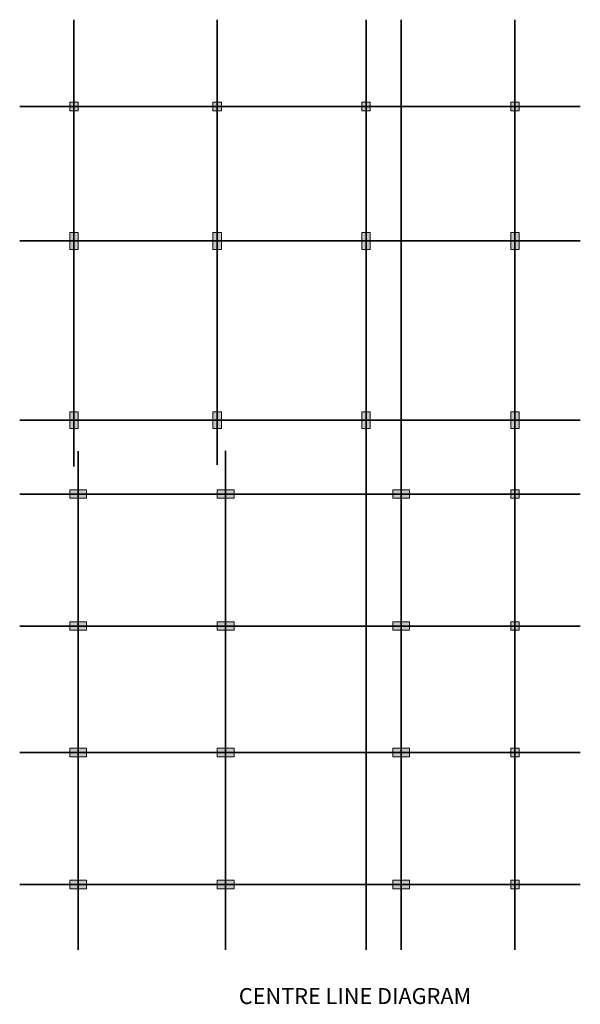
# Model space of a CAD drawing. Units: inches. Extents: x 9239 to 26065, y 6728 to 14611.
# Tile 6 of 12: x 12020 to 12619, y 6917 to 7969. Entities that reach past the tile are written whole.
import ezdxf

# ---------------------------------------------------------------- set-up
doc = ezdxf.new("R2010")
doc.units = ezdxf.units.IN
doc.header["$MEASUREMENT"] = 0
doc.linetypes.add('CENTER', pattern=[50.8, 31.75, -6.35, 6.35, -6.35])
for name, color, linetype, lineweight in [('A-ANNO-TEXT', 7, 'Continuous', 18), ('A-GRID', 3, 'CENTER', 18), ('S-COLS', 1, 'Continuous', 35), ('S-PATT', 252, 'Continuous', 13)]:
    doc.layers.add(name, color=color, linetype=linetype, lineweight=lineweight)
doc.styles.get("Standard").update_dxf_attribs({"font": 'arial.ttf'})

msp = doc.modelspace()

# ---------------------------------------------------------------- hatches: boundary and pattern name
at = {"layer": 'S-PATT'}
h = msp.add_hatch(color=256, dxfattribs=at)
h.dxf.hatch_style = 1
h.paths.add_polyline_path([(12082.24, 7880.66), (12077.74, 7880.66), (12077.74, 7876.16), (12082.24, 7876.16)])
h.paths.add_polyline_path([(12077.74, 7880.66), (12073.24, 7880.66), (12073.24, 7876.16), (12077.74, 7876.16)])
h.paths.add_polyline_path([(12077.74, 7876.16), (12073.24, 7876.16), (12073.24, 7871.66), (12077.74, 7871.66)])
h.paths.add_polyline_path([(12082.24, 7876.16), (12077.74, 7876.16), (12077.74, 7871.66), (12082.24, 7871.66)])
h.paths.add_polyline_path([(12235.24, 7880.66), (12230.74, 7880.66), (12230.74, 7876.16), (12235.24, 7876.16)])
h.paths.add_polyline_path([(12235.24, 7876.16), (12230.74, 7876.16), (12230.74, 7871.66), (12235.24, 7871.66)])
h.paths.add_polyline_path([(12230.74, 7876.16), (12226.24, 7876.16), (12226.24, 7871.66), (12230.74, 7871.66)])
h.paths.add_polyline_path([(12230.74, 7880.66), (12226.24, 7880.66), (12226.24, 7876.16), (12230.74, 7876.16)])
h.paths.add_polyline_path([(12394.24, 7876.16), (12389.74, 7876.16), (12389.74, 7871.66), (12394.24, 7871.66)])
h.paths.add_polyline_path([(12394.24, 7880.66), (12389.74, 7880.66), (12389.74, 7876.16), (12394.24, 7876.16)])
h.paths.add_polyline_path([(12389.74, 7880.66), (12385.24, 7880.66), (12385.24, 7876.16), (12389.74, 7876.16)])
h.paths.add_polyline_path([(12389.74, 7876.16), (12385.24, 7876.16), (12385.24, 7871.66), (12389.74, 7871.66)])
h.paths.add_polyline_path([(12553.24, 7880.66), (12548.74, 7880.66), (12548.74, 7876.16), (12553.24, 7876.16)])
h.paths.add_polyline_path([(12548.74, 7880.66), (12544.24, 7880.66), (12544.24, 7876.16), (12548.74, 7876.16)])
h.paths.add_polyline_path([(12548.74, 7876.16), (12544.24, 7876.16), (12544.24, 7871.66), (12548.74, 7871.66)])
h.paths.add_polyline_path([(12553.24, 7876.16), (12548.74, 7876.16), (12548.74, 7871.66), (12553.24, 7871.66)])
h.paths.add_polyline_path([(12553.24, 7732.59), (12548.74, 7732.59), (12548.74, 7723.59), (12553.24, 7723.59)])
h.paths.add_polyline_path([(12553.24, 7741.59), (12548.74, 7741.59), (12548.74, 7732.59), (12553.24, 7732.59)])
h.paths.add_polyline_path([(12548.74, 7741.59), (12544.24, 7741.59), (12544.24, 7732.59), (12548.74, 7732.59)])
h.paths.add_polyline_path([(12548.74, 7732.59), (12544.24, 7732.59), (12544.24, 7723.59), (12548.74, 7723.59)])
h.paths.add_polyline_path([(12394.24, 7741.59), (12389.74, 7741.59), (12389.74, 7732.59), (12394.24, 7732.59)])
h.paths.add_polyline_path([(12389.74, 7741.59), (12385.24, 7741.59), (12385.24, 7732.59), (12389.74, 7732.59)])
h.paths.add_polyline_path([(12389.74, 7732.59), (12385.24, 7732.59), (12385.24, 7723.59), (12389.74, 7723.59)])
h.paths.add_polyline_path([(12394.24, 7732.59), (12389.74, 7732.59), (12389.74, 7723.59), (12394.24, 7723.59)])
h.paths.add_polyline_path([(12230.74, 7741.59), (12226.24, 7741.59), (12226.24, 7732.59), (12230.74, 7732.59)])
h.paths.add_polyline_path([(12235.24, 7741.59), (12230.74, 7741.59), (12230.74, 7732.59), (12235.24, 7732.59)])
h.paths.add_polyline_path([(12235.24, 7732.59), (12230.74, 7732.59), (12230.74, 7723.59), (12235.24, 7723.59)])
h.paths.add_polyline_path([(12230.74, 7732.59), (12226.24, 7732.59), (12226.24, 7723.59), (12230.74, 7723.59)])
h.paths.add_polyline_path([(12082.24, 7741.59), (12077.74, 7741.59), (12077.74, 7732.59), (12082.24, 7732.59)])
h.paths.add_polyline_path([(12077.74, 7741.59), (12073.24, 7741.59), (12073.24, 7732.59), (12077.74, 7732.59)])
h.paths.add_polyline_path([(12077.74, 7732.59), (12073.24, 7732.59), (12073.24, 7723.59), (12077.74, 7723.59)])
h.paths.add_polyline_path([(12082.24, 7732.59), (12077.74, 7732.59), (12077.74, 7723.59), (12082.24, 7723.59)])
h.paths.add_polyline_path([(12077.74, 7550.08), (12073.24, 7550.08), (12073.24, 7541.08), (12077.74, 7541.08)])
h.paths.add_polyline_path([(12082.24, 7550.08), (12077.74, 7550.08), (12077.74, 7541.08), (12082.24, 7541.08)])
h.paths.add_polyline_path([(12077.74, 7541.08), (12073.24, 7541.08), (12073.24, 7532.08), (12077.74, 7532.08)])
h.paths.add_polyline_path([(12082.24, 7541.08), (12077.74, 7541.08), (12077.74, 7532.08), (12082.24, 7532.08)])
h.paths.add_polyline_path([(12230.74, 7550.08), (12226.24, 7550.08), (12226.24, 7541.08), (12230.74, 7541.08)])
h.paths.add_polyline_path([(12235.24, 7550.08), (12230.74, 7550.08), (12230.74, 7541.08), (12235.24, 7541.08)])
h.paths.add_polyline_path([(12235.24, 7541.08), (12230.74, 7541.08), (12230.74, 7532.08), (12235.24, 7532.08)])
h.paths.add_polyline_path([(12230.74, 7541.08), (12226.24, 7541.08), (12226.24, 7532.08), (12230.74, 7532.08)])
h.paths.add_polyline_path([(12394.24, 7550.08), (12389.74, 7550.08), (12389.74, 7541.08), (12394.24, 7541.08)])
h.paths.add_polyline_path([(12389.74, 7550.08), (12385.24, 7550.08), (12385.24, 7541.08), (12389.74, 7541.08)])
h.paths.add_polyline_path([(12389.74, 7541.08), (12385.24, 7541.08), (12385.24, 7532.08), (12389.74, 7532.08)])
h.paths.add_polyline_path([(12394.24, 7541.08), (12389.74, 7541.08), (12389.74, 7532.08), (12394.24, 7532.08)])
h.paths.add_polyline_path([(12553.24, 7550.08), (12548.74, 7550.08), (12548.74, 7541.08), (12553.24, 7541.08)])
h.paths.add_polyline_path([(12548.74, 7550.08), (12544.24, 7550.08), (12544.24, 7541.08), (12548.74, 7541.08)])
h.paths.add_polyline_path([(12548.74, 7541.08), (12544.24, 7541.08), (12544.24, 7532.08), (12548.74, 7532.08)])
h.paths.add_polyline_path([(12553.24, 7541.08), (12548.74, 7541.08), (12548.74, 7532.08), (12553.24, 7532.08)])
h.paths.add_polyline_path([(12553.24, 7466.66), (12548.74, 7466.66), (12548.74, 7462.16), (12553.24, 7462.16)])
h.paths.add_polyline_path([(12553.24, 7462.16), (12548.74, 7462.16), (12548.74, 7457.66), (12553.24, 7457.66)])
h.paths.add_polyline_path([(12548.74, 7462.16), (12544.24, 7462.16), (12544.24, 7457.66), (12548.74, 7457.66)])
h.paths.add_polyline_path([(12548.74, 7466.66), (12544.24, 7466.66), (12544.24, 7462.16), (12548.74, 7462.16)])
h.paths.add_polyline_path([(12427.24, 7466.66), (12418.24, 7466.66), (12418.24, 7462.16), (12427.24, 7462.16)])
h.paths.add_polyline_path([(12436.24, 7466.66), (12427.24, 7466.66), (12427.24, 7462.16), (12436.24, 7462.16)])
h.paths.add_polyline_path([(12436.24, 7462.16), (12427.24, 7462.16), (12427.24, 7457.66), (12436.24, 7457.66)])
h.paths.add_polyline_path([(12427.24, 7462.16), (12418.24, 7462.16), (12418.24, 7457.66), (12427.24, 7457.66)])
h.paths.add_polyline_path([(12248.74, 7466.66), (12239.74, 7466.66), (12239.74, 7462.16), (12248.74, 7462.16)])
h.paths.add_polyline_path([(12239.74, 7466.66), (12230.74, 7466.66), (12230.74, 7462.16), (12239.74, 7462.16)])
h.paths.add_polyline_path([(12239.74, 7462.16), (12230.74, 7462.16), (12230.74, 7457.66), (12239.74, 7457.66)])
h.paths.add_polyline_path([(12248.74, 7462.16), (12239.74, 7462.16), (12239.74, 7457.66), (12248.74, 7457.66)])
h.paths.add_polyline_path([(12091.24, 7466.66), (12082.24, 7466.66), (12082.24, 7462.16), (12091.24, 7462.16)])
h.paths.add_polyline_path([(12082.24, 7466.66), (12073.24, 7466.66), (12073.24, 7462.16), (12082.24, 7462.16)])
h.paths.add_polyline_path([(12082.24, 7462.16), (12073.24, 7462.16), (12073.24, 7457.66), (12082.24, 7457.66)])
h.paths.add_polyline_path([(12091.24, 7462.16), (12082.24, 7462.16), (12082.24, 7457.66), (12091.24, 7457.66)])
h.paths.add_polyline_path([(12091.24, 7321.16), (12082.24, 7321.16), (12082.24, 7316.66), (12091.24, 7316.66)])
h.paths.add_polyline_path([(12091.24, 7325.66), (12082.24, 7325.66), (12082.24, 7321.16), (12091.24, 7321.16)])
h.paths.add_polyline_path([(12082.24, 7325.66), (12073.24, 7325.66), (12073.24, 7321.16), (12082.24, 7321.16)])
h.paths.add_polyline_path([(12082.24, 7321.16), (12073.24, 7321.16), (12073.24, 7316.66), (12082.24, 7316.66)])
h.paths.add_polyline_path([(12239.74, 7325.66), (12230.74, 7325.66), (12230.74, 7321.16), (12239.74, 7321.16)])
h.paths.add_polyline_path([(12248.74, 7325.66), (12239.74, 7325.66), (12239.74, 7321.16), (12248.74, 7321.16)])
h.paths.add_polyline_path([(12248.74, 7321.16), (12239.74, 7321.16), (12239.74, 7316.66), (12248.74, 7316.66)])
h.paths.add_polyline_path([(12239.74, 7321.16), (12230.74, 7321.16), (12230.74, 7316.66), (12239.74, 7316.66)])
h.paths.add_polyline_path([(12436.24, 7325.66), (12427.24, 7325.66), (12427.24, 7321.16), (12436.24, 7321.16)])
h.paths.add_polyline_path([(12427.24, 7325.66), (12418.24, 7325.66), (12418.24, 7321.16), (12427.24, 7321.16)])
h.paths.add_polyline_path([(12427.24, 7321.16), (12418.24, 7321.16), (12418.24, 7316.66), (12427.24, 7316.66)])
h.paths.add_polyline_path([(12436.24, 7321.16), (12427.24, 7321.16), (12427.24, 7316.66), (12436.24, 7316.66)])
h.paths.add_polyline_path([(12553.24, 7325.66), (12548.74, 7325.66), (12548.74, 7321.16), (12553.24, 7321.16)])
h.paths.add_polyline_path([(12548.74, 7321.16), (12544.24, 7321.16), (12544.24, 7316.66), (12548.74, 7316.66)])
h.paths.add_polyline_path([(12548.74, 7325.66), (12544.24, 7325.66), (12544.24, 7321.16), (12548.74, 7321.16)])
h.paths.add_polyline_path([(12553.24, 7321.16), (12548.74, 7321.16), (12548.74, 7316.66), (12553.24, 7316.66)])
h.paths.add_polyline_path([(12553.24, 7190.66), (12548.74, 7190.66), (12548.74, 7186.16), (12553.24, 7186.16)])
h.paths.add_polyline_path([(12548.74, 7190.66), (12544.24, 7190.66), (12544.24, 7186.16), (12548.74, 7186.16)])
h.paths.add_polyline_path([(12548.74, 7186.16), (12544.24, 7186.16), (12544.24, 7181.66), (12548.74, 7181.66)])
h.paths.add_polyline_path([(12553.24, 7186.16), (12548.74, 7186.16), (12548.74, 7181.66), (12553.24, 7181.66)])
h.paths.add_polyline_path([(12436.24, 7190.66), (12427.24, 7190.66), (12427.24, 7186.16), (12436.24, 7186.16)])
h.paths.add_polyline_path([(12427.24, 7190.66), (12418.24, 7190.66), (12418.24, 7186.16), (12427.24, 7186.16)])
h.paths.add_polyline_path([(12427.24, 7186.16), (12418.24, 7186.16), (12418.24, 7181.66), (12427.24, 7181.66)])
h.paths.add_polyline_path([(12436.24, 7186.16), (12427.24, 7186.16), (12427.24, 7181.66), (12436.24, 7181.66)])
h.paths.add_polyline_path([(12239.74, 7190.66), (12230.74, 7190.66), (12230.74, 7186.16), (12239.74, 7186.16)])
h.paths.add_polyline_path([(12248.74, 7190.66), (12239.74, 7190.66), (12239.74, 7186.16), (12248.74, 7186.16)])
h.paths.add_polyline_path([(12248.74, 7186.16), (12239.74, 7186.16), (12239.74, 7181.66), (12248.74, 7181.66)])
h.paths.add_polyline_path([(12239.74, 7186.16), (12230.74, 7186.16), (12230.74, 7181.66), (12239.74, 7181.66)])
h.paths.add_polyline_path([(12091.24, 7190.66), (12082.24, 7190.66), (12082.24, 7186.16), (12091.24, 7186.16)])
h.paths.add_polyline_path([(12082.24, 7190.66), (12073.24, 7190.66), (12073.24, 7186.16), (12082.24, 7186.16)])
h.paths.add_polyline_path([(12082.24, 7186.16), (12073.24, 7186.16), (12073.24, 7181.66), (12082.24, 7181.66)])
h.paths.add_polyline_path([(12091.24, 7186.16), (12082.24, 7186.16), (12082.24, 7181.66), (12091.24, 7181.66)])
h.paths.add_polyline_path([(12091.24, 7049.66), (12082.24, 7049.66), (12082.24, 7045.16), (12091.24, 7045.16)])
h.paths.add_polyline_path([(12091.24, 7045.16), (12082.24, 7045.16), (12082.24, 7040.66), (12091.24, 7040.66)])
h.paths.add_polyline_path([(12082.24, 7045.16), (12073.24, 7045.16), (12073.24, 7040.66), (12082.24, 7040.66)])
h.paths.add_polyline_path([(12082.24, 7049.66), (12073.24, 7049.66), (12073.24, 7045.16), (12082.24, 7045.16)])
h.paths.add_polyline_path([(12239.74, 7049.66), (12230.74, 7049.66), (12230.74, 7045.16), (12239.74, 7045.16)])
h.paths.add_polyline_path([(12248.74, 7049.66), (12239.74, 7049.66), (12239.74, 7045.16), (12248.74, 7045.16)])
h.paths.add_polyline_path([(12248.74, 7045.16), (12239.74, 7045.16), (12239.74, 7040.66), (12248.74, 7040.66)])
h.paths.add_polyline_path([(12239.74, 7045.16), (12230.74, 7045.16), (12230.74, 7040.66), (12239.74, 7040.66)])
h.paths.add_polyline_path([(12436.24, 7049.66), (12427.24, 7049.66), (12427.24, 7045.16), (12436.24, 7045.16)])
h.paths.add_polyline_path([(12436.24, 7045.16), (12427.24, 7045.16), (12427.24, 7040.66), (12436.24, 7040.66)])
h.paths.add_polyline_path([(12427.24, 7045.16), (12418.24, 7045.16), (12418.24, 7040.66), (12427.24, 7040.66)])
h.paths.add_polyline_path([(12427.24, 7049.66), (12418.24, 7049.66), (12418.24, 7045.16), (12427.24, 7045.16)])
h.paths.add_polyline_path([(12553.24, 7045.16), (12548.74, 7045.16), (12548.74, 7040.66), (12553.24, 7040.66)])
h.paths.add_polyline_path([(12553.24, 7049.66), (12548.74, 7049.66), (12548.74, 7045.16), (12553.24, 7045.16)])
h.paths.add_polyline_path([(12548.74, 7049.66), (12544.24, 7049.66), (12544.24, 7045.16), (12548.74, 7045.16)])
h.paths.add_polyline_path([(12548.74, 7045.16), (12544.24, 7045.16), (12544.24, 7040.66), (12548.74, 7040.66)])

# ---------------------------------------------------------------- linework, layer by layer
at = {"layer": 'A-GRID'}
for p, q in [((12073.24, 7880.66), (12082.24, 7880.66)), ((12073.24, 7871.66), (12073.24, 7880.66)), ((12082.24, 7880.66), (12082.24, 7871.66)), ((12226.24, 7880.66), (12235.24, 7880.66)), ((12226.24, 7871.66), (12226.24, 7880.66)), ((12235.24, 7880.66), (12235.24, 7871.66)), ((12385.24, 7880.66), (12394.24, 7880.66)), ((12385.24, 7871.66), (12385.24, 7880.66)), ((12394.24, 7880.66), (12394.24, 7871.66)), ((12544.24, 7880.66), (12553.24, 7880.66)), ((12544.24, 7871.66), (12544.24, 7880.66)), ((12553.24, 7880.66), (12553.24, 7871.66)), ((12082.24, 7871.66), (12073.24, 7871.66)), ((12226.24, 7871.66), (12235.24, 7871.66)), ((12235.24, 7871.66), (12226.24, 7871.66)), ((12385.24, 7871.66), (12394.24, 7871.66)), ((12394.24, 7871.66), (12385.24, 7871.66)), ((12553.24, 7871.66), (12544.24, 7871.66)), ((12073.24, 7741.59), (12082.24, 7741.59)), ((12073.24, 7723.59), (12073.24, 7741.59)), ((12082.24, 7741.59), (12082.24, 7723.59)), ((12226.24, 7741.59), (12235.24, 7741.59)), ((12226.24, 7723.59), (12226.24, 7741.59)), ((12235.24, 7741.59), (12235.24, 7723.59)), ((12385.24, 7741.59), (12394.24, 7741.59)), ((12385.24, 7723.59), (12385.24, 7741.59)), ((12394.24, 7741.59), (12394.24, 7723.59)), ((12544.24, 7741.59), (12553.24, 7741.59)), ((12544.24, 7723.59), (12544.24, 7741.59)), ((12553.24, 7741.59), (12553.24, 7723.59)), ((12082.24, 7723.59), (12073.24, 7723.59)), ((12235.24, 7723.59), (12226.24, 7723.59)), ((12394.24, 7723.59), (12385.24, 7723.59)), ((12553.24, 7723.59), (12544.24, 7723.59)), ((12073.24, 7550.08), (12082.24, 7550.08)), ((12073.24, 7532.08), (12073.24, 7550.08)), ((12082.24, 7550.08), (12082.24, 7532.08)), ((12226.24, 7550.08), (12235.24, 7550.08)), ((12226.24, 7532.08), (12226.24, 7550.08)), ((12235.24, 7550.08), (12235.24, 7532.08)), ((12385.24, 7550.08), (12394.24, 7550.08)), ((12385.24, 7532.08), (12385.24, 7550.08)), ((12394.24, 7550.08), (12394.24, 7532.08)), ((12544.24, 7550.08), (12553.24, 7550.08)), ((12544.24, 7532.08), (12544.24, 7550.08)), ((12553.24, 7550.08), (12553.24, 7532.08)), ((12082.24, 7532.08), (12073.24, 7532.08)), ((12235.24, 7532.08), (12226.24, 7532.08)), ((12394.24, 7532.08), (12385.24, 7532.08)), ((12553.24, 7532.08), (12544.24, 7532.08)), ((12073.24, 7457.66), (12073.24, 7466.66)), ((12073.24, 7466.66), (12091.24, 7466.66)), ((12091.24, 7457.66), (12073.24, 7457.66)), ((12091.24, 7466.66), (12091.24, 7457.66)), ((12230.74, 7457.66), (12230.74, 7466.66)), ((12230.74, 7466.66), (12248.74, 7466.66)), ((12248.74, 7457.66), (12230.74, 7457.66)), ((12248.74, 7466.66), (12248.74, 7457.66)), ((12418.24, 7457.66), (12418.24, 7466.66)), ((12418.24, 7466.66), (12436.24, 7466.66)), ((12436.24, 7457.66), (12418.24, 7457.66)), ((12436.24, 7466.66), (12436.24, 7457.66)), ((12544.24, 7466.66), (12553.24, 7466.66)), ((12544.24, 7457.66), (12544.24, 7466.66)), ((12553.24, 7457.66), (12544.24, 7457.66)), ((12553.24, 7466.66), (12553.24, 7457.66)), ((12073.24, 7316.66), (12073.24, 7325.66)), ((12073.24, 7325.66), (12091.24, 7325.66)), ((12091.24, 7325.66), (12091.24, 7316.66)), ((12230.74, 7316.66), (12230.74, 7325.66)), ((12230.74, 7325.66), (12248.74, 7325.66)), ((12248.74, 7325.66), (12248.74, 7316.66)), ((12418.24, 7316.66), (12418.24, 7325.66)), ((12418.24, 7325.66), (12436.24, 7325.66)), ((12436.24, 7325.66), (12436.24, 7316.66)), ((12544.24, 7325.66), (12553.24, 7325.66)), ((12544.24, 7316.66), (12544.24, 7325.66)), ((12553.24, 7325.66), (12553.24, 7316.66)), ((12091.24, 7316.66), (12073.24, 7316.66)), ((12248.74, 7316.66), (12230.74, 7316.66)), ((12436.24, 7316.66), (12418.24, 7316.66)), ((12553.24, 7316.66), (12544.24, 7316.66)), ((12073.24, 7181.66), (12073.24, 7190.66)), ((12073.24, 7190.66), (12091.24, 7190.66)), ((12091.24, 7190.66), (12091.24, 7181.66)), ((12230.74, 7181.66), (12230.74, 7190.66)), ((12230.74, 7190.66), (12248.74, 7190.66)), ((12248.74, 7190.66), (12248.74, 7181.66)), ((12418.24, 7181.66), (12418.24, 7190.66)), ((12418.24, 7190.66), (12436.24, 7190.66)), ((12436.24, 7190.66), (12436.24, 7181.66)), ((12544.24, 7190.66), (12553.24, 7190.66)), ((12544.24, 7181.66), (12544.24, 7190.66)), ((12553.24, 7190.66), (12553.24, 7181.66)), ((12091.24, 7181.66), (12073.24, 7181.66)), ((12248.74, 7181.66), (12230.74, 7181.66)), ((12436.24, 7181.66), (12418.24, 7181.66)), ((12553.24, 7181.66), (12544.24, 7181.66)), ((12073.24, 7040.66), (12073.24, 7049.66)), ((12073.24, 7049.66), (12091.24, 7049.66)), ((12091.24, 7049.66), (12091.24, 7040.66)), ((12230.74, 7040.66), (12230.74, 7049.66)), ((12230.74, 7049.66), (12248.74, 7049.66)), ((12248.74, 7049.66), (12248.74, 7040.66)), ((12418.24, 7040.66), (12418.24, 7049.66)), ((12418.24, 7049.66), (12436.24, 7049.66)), ((12427.24, 7049.66), (12436.24, 7049.66)), ((12436.24, 7049.66), (12436.24, 7040.66)), ((12544.24, 7049.66), (12553.24, 7049.66)), ((12544.24, 7040.66), (12544.24, 7049.66)), ((12553.24, 7049.66), (12553.24, 7040.66)), ((12091.24, 7040.66), (12073.24, 7040.66)), ((12248.74, 7040.66), (12230.74, 7040.66)), ((12436.24, 7040.66), (12418.24, 7040.66)), ((12553.24, 7040.66), (12544.24, 7040.66))]:
    msp.add_line(p, q, dxfattribs=at)
at = {"layer": 'S-COLS'}
for p, q in [((12077.74, 7968.88), (12077.74, 7491.5)), ((12230.74, 7968.88), (12230.74, 7493.51)), ((12389.74, 7968.88), (12389.74, 6975.27)), ((12427.24, 6975.27), (12427.24, 7968.88)), ((12548.74, 7968.88), (12548.74, 6975.27)), ((12077.74, 7880.66), (12077.74, 7871.66)), ((12230.74, 7880.66), (12230.74, 7871.66)), ((12389.74, 7880.66), (12389.74, 7871.66)), ((12548.74, 7880.66), (12548.74, 7871.66)), ((12019.82, 7876.16), (12618.59, 7876.16)), ((12073.24, 7876.16), (12082.24, 7876.16)), ((12226.24, 7876.16), (12235.24, 7876.16)), ((12385.24, 7876.16), (12394.24, 7876.16)), ((12544.24, 7876.16), (12553.24, 7876.16)), ((12077.74, 7741.59), (12077.74, 7723.59)), ((12230.74, 7741.59), (12230.74, 7723.59)), ((12389.74, 7741.59), (12389.74, 7723.59)), ((12548.74, 7741.59), (12548.74, 7723.59)), ((12019.82, 7732.59), (12618.59, 7732.59)), ((12019.82, 7541.08), (12618.59, 7541.08)), ((12077.74, 7550.08), (12077.74, 7532.08)), ((12230.74, 7550.08), (12230.74, 7532.08)), ((12389.74, 7550.08), (12389.74, 7532.08)), ((12548.74, 7550.08), (12548.74, 7532.08)), ((12082.24, 7508.1), (12082.24, 6975.27)), ((12239.74, 7508.28), (12239.74, 6975.27)), ((12019.82, 7462.16), (12618.59, 7462.16)), ((12091.24, 7462.16), (12073.24, 7462.16)), ((12248.74, 7462.16), (12230.74, 7462.16)), ((12436.24, 7462.16), (12418.24, 7462.16)), ((12544.24, 7462.16), (12553.24, 7462.16)), ((12548.74, 7466.66), (12548.74, 7457.66)), ((12019.82, 7321.16), (12618.59, 7321.16)), ((12091.24, 7321.16), (12073.24, 7321.16)), ((12248.74, 7321.16), (12230.74, 7321.16)), ((12436.24, 7321.16), (12418.24, 7321.16)), ((12544.24, 7321.16), (12553.24, 7321.16)), ((12548.74, 7325.66), (12548.74, 7316.66)), ((12019.82, 7186.16), (12618.59, 7186.16)), ((12091.24, 7186.16), (12073.24, 7186.16)), ((12248.74, 7186.16), (12230.74, 7186.16)), ((12436.24, 7186.16), (12418.24, 7186.16)), ((12544.24, 7186.16), (12553.24, 7186.16)), ((12548.74, 7190.66), (12548.74, 7181.66)), ((12548.74, 7049.66), (12548.74, 7040.66)), ((12019.82, 7045.16), (12618.59, 7045.16)), ((12091.24, 7045.16), (12073.24, 7045.16)), ((12248.74, 7045.16), (12230.74, 7045.16)), ((12436.24, 7045.16), (12418.24, 7045.16)), ((12544.24, 7045.16), (12553.24, 7045.16))]:
    msp.add_line(p, q, dxfattribs=at)

# ---------------------------------------------------------------- texts
at = {"layer": 'A-ANNO-TEXT', "insert": (12253.88, 6934.52), "char_height": 17, "attachment_point": 1}
msp.add_mtext_dynamic_manual_height_columns('CENTRE LINE DIAGRAM', width=2149.001, gutter_width=1, heights=[0], dxfattribs=at)

doc.saveas('drawing.dxf')
